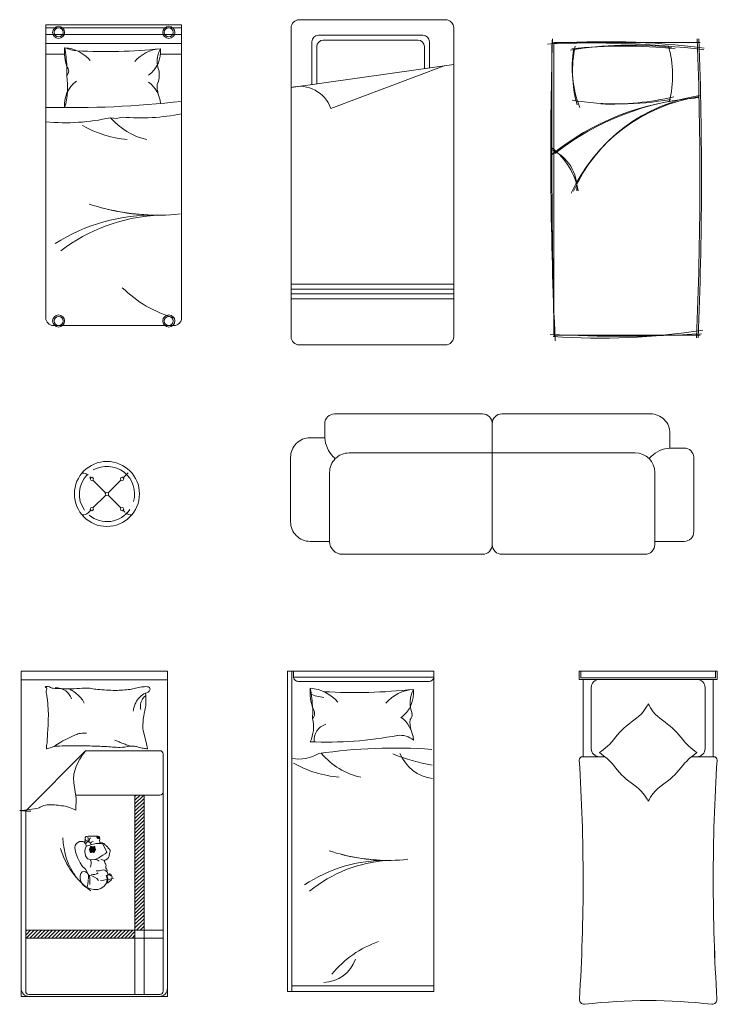
# Model space of a CAD drawing. Units: inches. Extents: x -17 to 1735, y -531 to 60.
# Tile 27 of 27: x 1734.8647 to 1735.0336, y -150.4015 to -150.163. Entities that reach past the tile are written whole.
import ezdxf

# ---------------------------------------------------------------- set-up
doc = ezdxf.new("R2010")
doc.units = ezdxf.units.IN
doc.header["$MEASUREMENT"] = 0
doc.layers.add('A-FURN', color=242, linetype='Continuous', lineweight=18, true_color=0xcd2027)
pattern_1 = [(315, (86.7872822, 39.0477945), (0.00194454365, 0.00194454365), [])]

# ---------------------------------------------------------------- blocks, each defined once
blk = doc.blocks.new('childrens_room_2')
h = blk.add_hatch()
h.set_pattern_fill('ANSI31', color=256, scale=0.005, angle=-90, style=0)
h.set_pattern_definition([(45, (74.756955, 52.19314), (-0.01122532, 0.01122532), [])])
h.paths.add_polyline_path([(75.7484, 49.9124), (75.6924, 49.9124), (75.6924, 50.7433), (75.7484, 50.7433)])
h.paths.add_polyline_path([(75.6924, 49.9124), (75.6924, 49.8634), (75.0203, 49.8634), (75.0203, 49.9124)])
h = blk.add_hatch()
h.set_pattern_fill('ANSI31', color=256, scale=0.022, angle=-90, style=0)
h.set_pattern_definition(pattern_1)
h.paths.add_polyline_path([(75.4756, 50.4754), (75.4753, 50.4804), (75.4736, 50.4848), (75.4694, 50.4881), (75.4661, 50.4896), (75.4574, 50.4905, 0.479357)])
h = blk.add_hatch()
h.set_pattern_fill('ANSI31', color=256, scale=0.022, angle=-90, style=0)
h.set_pattern_definition(pattern_1)
h.paths.add_polyline_path([(75.4157, 50.4038), (75.4153, 50.3984), (75.4172, 50.3931), (75.4208, 50.39), (75.425, 50.39), (75.431, 50.3928), (75.4354, 50.3938), (75.4375, 50.3921), (75.4403, 50.3907), (75.4436, 50.3921), (75.4442, 50.3948), (75.4443, 50.3978), (75.4455, 50.4018), (75.4489, 50.407), (75.4494, 50.4084), (75.446, 50.4144), (75.445, 50.417), (75.4457, 50.4212), (75.4461, 50.4241), (75.4435, 50.4269), (75.4407, 50.4259), (75.4383, 50.4231), (75.4332, 50.4237), (75.4242, 50.4273), (75.4199, 50.4264), (75.4193, 50.4235), (75.4187, 50.4213), (75.4164, 50.4195), (75.4165, 50.4173), (75.4153, 50.4135), (75.4128, 50.4109), (75.4115, 50.4095), (75.4136, 50.4078)])
for p, q in [((75.9793, 55.4814), (75.144, 55.4814)), ((75.144, 55.4814), (75.144, 53.6781)), ((75.9793, 55.4814), (75.9793, 53.6781)), ((76.7025, 55.5128), (77.6025, 55.5128)), ((75.9793, 55.4628), (75.144, 55.4628)), ((75.9793, 55.4225), (75.144, 55.4225)), ((76.6525, 53.5628), (76.6525, 55.4628)), ((77.6525, 53.5628), (77.6525, 55.4628)), ((75.9793, 55.3673), (75.144, 55.3673)), ((76.7804, 55.3772), (76.7804, 55.1146)), ((77.4628, 55.4172), (76.8204, 55.4172)), ((77.4328, 55.3872), (76.8504, 55.3872)), ((77.5028, 55.2164), (77.5028, 55.3772)), ((78.2687, 55.3728), (79.1687, 55.3728)), ((78.2687, 53.5728), (78.2687, 55.3728)), ((75.2595, 55.3013), (75.144, 55.3013)), ((75.9793, 55.3013), (75.8487, 55.3013)), ((76.8104, 55.3472), (76.8104, 55.1188)), ((77.4728, 55.2122), (77.4728, 55.3472)), ((77.6525, 55.2375), (76.6525, 55.0966)), ((76.8961, 54.9672), (77.5948, 55.2294)), ((76.6525, 53.8862), (77.6525, 53.8862)), ((76.6525, 53.8562), (77.6525, 53.8562)), ((76.6525, 53.8262), (77.6525, 53.8262)), ((76.6525, 53.7962), (77.6525, 53.7962)), ((75.1904, 53.6317), (75.9329, 53.6317)), ((79.1687, 53.5728), (78.2687, 53.5728)), ((77.6025, 53.5128), (76.7025, 53.5128)), ((76.8595, 53.0278), (76.8595, 52.941)), ((77.8894, 53.0282), (77.8894, 52.2842)), ((77.8894, 52.2842), (77.8894, 53.0282)), ((76.8599, 52.941), (76.7694, 52.941)), ((78.9826, 52.8777), (78.9826, 52.9682)), ((76.9245, 52.8126), (76.9123, 52.8249)), ((77.0094, 52.8478), (77.8894, 52.8482)), ((77.8894, 52.8482), (78.7694, 52.8482)), ((78.8542, 52.813), (78.8665, 52.8253)), ((75.4201, 52.6953), (75.4145, 52.7009)), ((75.6201, 52.6953), (75.6509, 52.7262)), ((76.8894, 52.3038), (76.8894, 52.7278)), ((78.8894, 52.7282), (78.8894, 52.3038)), ((75.51, 52.6054), (75.4343, 52.6812)), ((75.5272, 52.6024), (75.6059, 52.6812)), ((75.4343, 52.5095), (75.513, 52.5883)), ((75.6059, 52.5095), (75.5301, 52.5853)), ((75.4046, 52.4798), (75.4201, 52.4954)), ((75.631, 52.4844), (75.6201, 52.4954)), ((76.7694, 52.3038), (76.8894, 52.3038)), ((78.8894, 52.2842), (78.8894, 52.3038)), ((77.4337, 52.2242), (77.4534, 52.2242)), ((74.9919, 51.5044), (74.9919, 49.5044)), ((75.8919, 51.5044), (74.9919, 51.5044)), ((75.8919, 49.5044), (75.8919, 51.5044)), ((76.6309, 49.5344), (76.6309, 51.5044)), ((76.6309, 51.5044), (77.5309, 51.5044)), ((76.6579, 49.5344), (76.6579, 51.5044)), ((77.5309, 51.5044), (77.5309, 49.5344)), ((75.8919, 51.452), (74.9919, 51.452)), ((76.6669, 51.4694), (77.5309, 51.4694)), ((78.4985, 51.4044), (78.4985, 51.0294)), ((79.1985, 51.4044), (79.1985, 51.0294)), ((75.3892, 51.0159), (75.0203, 50.6461)), ((75.3892, 51.0159), (75.8461, 51.0159)), ((75.8661, 50.9959), (75.8661, 49.5366)), ((78.4449, 50.9794), (78.582, 50.9794)), ((79.1151, 50.9794), (79.2522, 50.9794)), ((75.8461, 50.7433), (75.3274, 50.7433)), ((75.0203, 49.5366), (75.0203, 50.6461)), ((75.8661, 49.9124), (75.0203, 49.9124)), ((75.8661, 49.8634), (75.0203, 49.8634)), ((77.5309, 49.5694), (76.6579, 49.5694)), ((74.9919, 49.5044), (75.8919, 49.5044)), ((75.8461, 49.5166), (75.0403, 49.5166)), ((77.5309, 49.5344), (76.6309, 49.5344))]:
    blk.add_line(p, q)
for points in [[(75.144, 54.8843, 0.078314), (75.5425, 54.9102, 0.174082), (75.6138, 54.9142, 0.074189), (75.9793, 54.9344)], [(78.8294, 52.2242), (77.9494, 52.2242, -0.414214), (77.8894, 52.2842, -0.414214), (77.8294, 52.2242), (77.4534, 52.2242), (77.4534, 52.2242, -0.414214), (77.4534, 52.2242), (76.9678, 52.2242, -0.404299), (76.8894, 52.3038), (76.7694, 52.3038, -0.414214), (76.6494, 52.4238), (76.6494, 52.821, -0.414214), (76.7694, 52.941), (76.8595, 52.941), (76.8595, 53.0278, -0.409533), (76.9195, 53.0882), (77.8294, 53.0882, -0.414482), (77.8894, 53.0282, -0.414214), (77.9494, 53.0882), (78.8626, 53.0882, -0.414214), (78.9826, 52.9682), (78.9826, 52.878), (79.0694, 52.878, -0.394315), (79.1292, 52.8221), (79.1294, 52.3638, -0.41421), (79.0694, 52.3038), (78.8894, 52.3038), (78.8894, 52.2842, -0.414214), (78.8294, 52.2242, -2.414214)], [(76.6669, 51.5044), (76.6669, 51.4726, 0.414214), (76.6969, 51.4426), (77.5009, 51.4426, 0.414214), (77.5309, 51.4726)], [(79.2522, 50.9794), (79.2485, 50.9794), (79.2485, 51.4544), (79.2735, 51.4544), (79.2735, 51.5044), (78.4235, 51.5044), (78.4235, 51.4544), (78.4485, 51.4544), (78.4485, 50.9794), (78.4449, 50.9794, 0.433007), (78.4249, 50.9581, -0.031616), (78.4257, 49.4879, 0.44677), (78.457, 49.456, -0.059749), (79.24, 49.456, 0.44677), (79.2714, 49.4879, -0.031616), (79.2722, 50.9581, 0.433007), (79.2522, 50.9794), (79.2485, 50.9794)], [(75.7568, 51.3708, 0.263368), (75.7848, 51.3896, 0.494818), (75.7756, 51.4083, 0.049225), (75.7579, 51.4101, 0.036831), (75.7343, 51.4083, 0.031893), (75.6963, 51.4002, -0.035782), (75.6624, 51.3932, -0.032941), (75.5727, 51.3873, -0.026564), (75.4615, 51.3932, -0.017905), (75.424, 51.3986, 0.033397), (75.4038, 51.4008, 0.03204), (75.3667, 51.4001, -0.018442), (75.3024, 51.3971, -0.010837), (75.2376, 51.3978, -0.014624), (75.1897, 51.4008, -0.111249), (75.1671, 51.4081, 0.153708), (75.1503, 51.4121, 0.076444), (75.1428, 51.4104, 0.215512), (75.1409, 51.4083, 0.585858), (75.1435, 51.4053, -0.363489), (75.1484, 51.4027, -0.191716), (75.1484, 51.3912, 0.129675), (75.1465, 51.3746, 0.01735), (75.1495, 51.3577, -0.019326), (75.1521, 51.3427, -0.018818), (75.1587, 51.2743, -0.021828), (75.1596, 51.215, -0.006204), (75.1583, 51.1812, -0.001963), (75.1521, 51.0743, -0.028341), (75.1479, 51.0382, 0.117014), (75.1484, 51.0293, 0.36606), (75.1498, 51.0283, 0.03973), (75.1634, 51.0311, 0.048309), (75.1771, 51.0366, -0.062981), (75.1878, 51.0405, -0.04058), (75.2112, 51.0439, -0.014345), (75.2779, 51.0461, -0.005484), (75.4034, 51.0454, -0.007153), (75.4995, 51.0424, -0.008762), (75.5421, 51.0397, 0.008153), (75.5878, 51.0368, 0.06251), (75.6449, 51.0412, -0.078669), (75.6905, 51.0432, -0.047825), (75.7129, 51.0385, 0.034494), (75.7437, 51.0311, 0.023571), (75.769, 51.0281, 0.510228), (75.7699, 51.0293), (75.7624, 51.0593), (75.7418, 51.1419, -0.073041), (75.7398, 51.1614, -0.023305), (75.7455, 51.2225, -0.018299), (75.7496, 51.2454, 0.01097), (75.7569, 51.2834, 0.042281), (75.7599, 51.3177, 0.027201), (75.7569, 51.3711)], [(75.201, 51.4027, -0.088153), (75.2355, 51.3992, -0.088153), (75.2667, 51.3839, -0.077547), (75.2883, 51.3623, -0.077547), (75.3024, 51.3351)], [(75.2829, 51.397, -0.027842), (75.3067, 51.3864, -0.048685), (75.3193, 51.3783, -0.023666), (75.3472, 51.3539, -0.031223), (75.3662, 51.3333, -0.046801), (75.3713, 51.3256, -0.023191), (75.3794, 51.3089)], [(75.757, 51.3708, 0.077379), (75.7222, 51.3455, 0.077379), (75.6967, 51.3107, 0.047525), (75.6868, 51.2861, 0.047525), (75.6817, 51.2601)], [(75.7585, 51.3548, 0.05369), (75.7442, 51.3418, 0.070312), (75.7361, 51.3295, 0.015448), (75.7324, 51.321, 0.013244), (75.7286, 51.3107, 0.082127), (75.7256, 51.2927, 0.064164), (75.7286, 51.2695)], [(75.1972, 51.0424, -0.016108), (75.2361, 51.0686, -0.024599), (75.2629, 51.0837, -0.009477), (75.312, 51.107, -0.015937), (75.3418, 51.1193, -0.072521), (75.3581, 51.1229, -0.033339), (75.3944, 51.1231)], [(75.6664, 51.0439, -0.009729), (75.6391, 51.053, -0.009729), (75.6122, 51.063, -0.007971), (75.5905, 51.0721, -0.007971), (75.569, 51.0818)], [(75.3892, 51.0159, 0.085272), (75.3259, 50.9058, 0.124044), (75.3167, 50.8182), (75.3304, 50.7228), (75.3286, 50.6503)], [(76.6579, 50.9684, 0.174518), (76.8222, 50.998, -0.055694), (77.517, 51.0241)], [(75.3286, 50.6503, 0.027362), (75.2901, 50.6667, 0.040834), (75.2629, 50.6741, 0.038441), (75.1753, 50.6837, 0.076528), (75.1312, 50.6783, 0.103649), (75.1036, 50.6639, -0.026469), (74.9835, 50.6474, -0.024037), (75.0514, 50.6436, -0.052315), (75.0203, 50.6461)]]:
    blk.add_lwpolyline(points, format="xyb")
for points in [[(78.4235, 51.4544), (79.2735, 51.4544), (79.2735, 51.5044), (78.4235, 51.5044)], [(78.4335, 51.4644), (79.2635, 51.4644), (79.2635, 51.5044), (78.4335, 51.5044)]]:
    blk.add_lwpolyline(points, close=True)
for points in [[(79.2485, 50.9794), (79.2485, 51.4544), (78.4485, 51.4544), (78.4485, 50.9794)], [(75.6924, 49.5166), (75.6924, 50.7433)], [(75.7484, 49.5166), (75.7484, 50.7433)], [(75.4495, 50.4907), (75.436, 50.4914), (75.4203, 50.4904), (75.4036, 50.4898), (75.3986, 50.4892), (75.3926, 50.4889), (75.3864, 50.4823), (75.386, 50.476), (75.3873, 50.4713), (75.3842, 50.4665), (75.3854, 50.4621), (75.382, 50.454), (75.3779, 50.4546), (75.3722, 50.4577), (75.3521, 50.4571), (75.3405, 50.4511), (75.3333, 50.4449), (75.3254, 50.4326), (75.3235, 50.4197), (75.3264, 50.3946), (75.338, 50.359), (75.3556, 50.3273), (75.3703, 50.3034), (75.3857, 50.2905), (75.3892, 50.288), (75.3989, 50.2691), (75.3992, 50.2672), (75.3974, 50.2654), (75.3879, 50.2716), (75.381, 50.2735), (75.3675, 50.272), (75.3603, 50.2613), (75.3555, 50.2467), (75.3548, 50.229), (75.3596, 50.2113), (75.3725, 50.1916), (75.3908, 50.176), (75.4017, 50.1719), (75.4078, 50.1712), (75.4214, 50.1658), (75.4397, 50.1631), (75.4642, 50.1631), (75.4832, 50.1685), (75.5022, 50.1835), (75.5165, 50.2018), (75.526, 50.2039), (75.547, 50.2188), (75.5518, 50.2372), (75.5443, 50.2569), (75.5375, 50.2582), (75.5308, 50.2525), (75.5289, 50.252), (75.5261, 50.2586), (75.5239, 50.263), (75.5228, 50.2642), (75.5217, 50.27), (75.5203, 50.2719), (75.5214, 50.2813), (75.5169, 50.2902), (75.5139, 50.293), (75.5136, 50.3049), (75.515, 50.3102), (75.5106, 50.3204), (75.5086, 50.3215), (75.5078, 50.3309), (75.5039, 50.3376), (75.5061, 50.342), (75.5128, 50.3453), (75.5233, 50.3506), (75.5305, 50.3589), (75.5327, 50.3678), (75.5344, 50.3728), (75.5349, 50.3805), (75.5361, 50.3864), (75.5394, 50.3933), (75.5408, 50.3972), (75.5405, 50.4041), (75.5336, 50.4127), (75.5297, 50.4138), (75.5264, 50.4215), (75.5233, 50.426), (75.5194, 50.4274), (75.5175, 50.4296), (75.5158, 50.4321), (75.51, 50.4348), (75.5086, 50.436), (75.5086, 50.4379), (75.5031, 50.4432), (75.5006, 50.4457), (75.4962, 50.4454), (75.4917, 50.449), (75.4879, 50.4487), (75.4807, 50.4493), (75.4773, 50.4501), (75.476, 50.4509), (75.4766, 50.4526), (75.4769, 50.4574), (75.4751, 50.461), (75.4749, 50.4631), (75.4758, 50.4719), (75.4753, 50.4804), (75.4736, 50.4848), (75.4694, 50.4881), (75.4661, 50.4896), (75.4532, 50.4909), (75.4495, 50.4907)], [(75.4954, 50.4409), (75.5077, 50.4188), (75.5192, 50.3914), (75.5099, 50.3825), (75.494, 50.3728), (75.4662, 50.3551), (75.4463, 50.3472), (75.4251, 50.345), (75.4004, 50.3512), (75.3889, 50.3693), (75.384, 50.3954), (75.3863, 50.4148), (75.3942, 50.4289), (75.4269, 50.4387), (75.453, 50.4444), (75.4803, 50.4453), (75.4954, 50.4409)], [(75.4494, 50.4084), (75.446, 50.4144), (75.445, 50.417), (75.4457, 50.4212), (75.4461, 50.4241), (75.4435, 50.4269), (75.4407, 50.4259), (75.4383, 50.4231), (75.4332, 50.4237), (75.4242, 50.4273), (75.4199, 50.4264), (75.4193, 50.4235), (75.4187, 50.4213), (75.4164, 50.4195), (75.4165, 50.4173), (75.4153, 50.4135), (75.4128, 50.4109), (75.4115, 50.4095), (75.4136, 50.4078), (75.4157, 50.4038), (75.4153, 50.3984), (75.4172, 50.3931), (75.4208, 50.39), (75.425, 50.39), (75.431, 50.3928), (75.4354, 50.3938), (75.4375, 50.3921), (75.4403, 50.3907), (75.4436, 50.3921), (75.4442, 50.3948), (75.4443, 50.3978), (75.4455, 50.4018), (75.4489, 50.407), (75.4494, 50.4084)]]:
    blk.add_lwpolyline(points)
for centre, radius in [((75.2229, 55.435), 0.0371), ((75.2229, 55.435), 0.0278), ((75.9004, 55.435), 0.0371), ((75.9004, 55.435), 0.0278), ((75.2229, 53.6596), 0.0371), ((75.2229, 53.6596), 0.0278), ((75.9004, 53.6596), 0.0371), ((75.9004, 53.6596), 0.0278), ((75.5201, 52.5954), 0.2), ((75.4272, 52.6883), 0.01), ((75.613, 52.6883), 0.01), ((75.5201, 52.5954), 0.01), ((75.4272, 52.5025), 0.01), ((75.613, 52.5025), 0.01)]:
    blk.add_circle(centre, radius)
for centre, radius, start, end in [((76.7025, 55.4628), 0.05, 90, 180), ((77.6025, 55.4628), 0.05, 0, 90), ((76.8204, 55.3772), 0.04, 90, 180), ((76.8504, 55.3472), 0.04, 90, 180), ((77.4328, 55.3472), 0.04, 0, 90), ((77.4628, 55.3772), 0.04, 0, 90), ((78.5913, 50.8189), 4.5588, 82.42637, 94.55161), ((78.5011, 49.6503), 5.7195, 83.0717, 92.72063), ((102.953, 54.6963), 24.7034, 178.37753, 182.68762), ((142.1352, 54.9109), 63.8797, 179.573644, 181.208723), ((56.1732, 54.5417), 22.9932, 357.54182, 2.12882), ((56.1732, 54.5417), 23.0032, 357.54182, 2.12882), ((75.5453, 55.3172), 0.2863, 175.30484, 198.69419), ((75.3647, 55.5935), 0.2736, 247.51785, 264.26696), ((75.2441, 55.1139), 0.2274, 40.4189, 85.9871), ((73.7608, 55.0981), 1.5188, 4.80985, 9.18918), ((75.5117, 58.4538), 3.1374, 266.81337, 276.16021), ((75.8643, 55.1077), 0.2274, 94.0129, 139.5811), ((75.669, 55.316), 0.1804, 306.5711, 5.88998), ((75.9929, 55.2569), 0.164, 151.77364, 201.69827), ((78.7416, 53.0702), 2.286, 83.69688, 99.35881), ((78.6932, 52.3041), 3.0464, 83.94088, 95.93515), ((79.0436, 55.2168), 0.6622, 169.79049, 201.55888), ((79.1653, 55.1958), 0.7819, 168.56961, 195.27012), ((78.3558, 55.1693), 0.6428, 345.48198, 16.58826), ((75.2435, 55.1977), 0.0414, 314.4736, 42.17134), ((73.0827, 55.2679), 2.1921, 357.39054, 358.88764), ((75.6858, 55.1758), 0.156, 337.01696, 7.53676), ((75.4394, 54.9904), 0.1804, 126.5711, 185.88998), ((74.8178, 55.0985), 0.46, 344.0243, 8.70709), ((75.669, 54.9843), 0.1804, 4.31813, 53.4289), ((75.9991, 55.1007), 0.1702, 175.22328, 196.23004), ((76.7043, 54.9001), 0.2032, 19.27951, 104.76299), ((75.2957, 61.0539), 6.082, 268.57082, 276.45367), ((79.2465, 53.4559), 1.5775, 94.14563, 129.02089), ((79.2814, 53.412), 1.6265, 94.18593, 128.21496), ((79.3165, 54.015), 1.0355, 98.91724, 155.46246), ((78.6697, 56.7642), 1.7696, 260.58531, 280.2821), ((79.3129, 54.0449), 1.0119, 98.39844, 155.88807), ((78.6184, 56.6764), 1.6826, 267.95445, 283.33938), ((75.5045, 53.3317), 1.6584, 97.85852, 98.47626), ((75.2441, 55.1987), 0.2274, 274.0129, 278.34166), ((75.8605, 55.1841), 0.4198, 220.73328, 256.96719), ((75.7087, 55.4543), 0.6823, 240.14078, 264.51099), ((78.1507, 54.4748), 0.2599, 356.64662, 66.65295), ((77.9988, 54.3854), 0.4254, 10.16482, 52.268), ((75.8487, 55.7499), 1.4398, 252.27047, 269.13024), ((75.8269, 55.5836), 1.2733, 255.03258, 276.43831), ((75.8025, 53.1895), 1.1211, 88.75448, 122.44857), ((75.8891, 53.2381), 1.074, 93.31876, 127.41471), ((76.1443, 54.4045), 0.7565, 225.55548, 253.7707), ((75.1904, 53.6781), 0.0464, 180, 270), ((75.9329, 53.6781), 0.0464, 270, 0), ((78.5471, 57.6422), 4.0883, 266.02934, 278.96409), ((76.7025, 53.5628), 0.05, 180, 270), ((77.6025, 53.5628), 0.05, 270, 0), ((78.6779, 61.5696), 8.0041, 266.89864, 273.56403), ((75.5201, 52.5954), 0.17, 344.03296, 119.71985), ((75.5201, 52.5954), 0.17, 135.42029, 215.97163), ((75.3738, 52.6824), 0.0419, 42.82742, 99.74562), ((75.503, 52.6011), 0.0083, 347.80192, 31.53697), ((75.5396, 52.5905), 0.0108, 179.91033, 208.61328), ((75.3738, 52.5083), 0.0419, 260.25438, 317.17258), ((75.5201, 52.5954), 0.17, 229.841, 326.08002), ((75.6664, 52.5083), 0.0419, 222.82742, 279.74562), ((78.5485, 51.4044), 0.05, 90, 180), ((79.1485, 51.4044), 0.05, 0, 90), ((77.0781, 51.3748), 0.3085, 175.30484, 198.69419), ((75.1553, 51.1387), 1.6364, 4.80985, 9.18918), ((76.7535, 51.1557), 0.245, 40.4189, 85.9871), ((76.8834, 51.6374), 0.2948, 247.51785, 264.26696), ((77.0419, 54.7542), 3.3803, 266.81337, 276.16021), ((77.4217, 51.149), 0.245, 94.0129, 139.5811), ((77.2113, 51.3735), 0.1943, 306.5711, 5.88998), ((77.5603, 51.3098), 0.1767, 151.77364, 201.69827), ((76.7528, 51.246), 0.0446, 314.4736, 42.17134), ((74.4247, 51.3217), 2.3618, 357.39054, 358.88764), ((77.3634, 51.2349), 0.034, 307.61433, 16.28017), ((76.5848, 51.1619), 0.206, 333.80176, 14.68402), ((77.2113, 51.0672), 0.1943, 4.31813, 53.4289), ((77.5669, 51.1927), 0.1834, 175.22328, 196.23004), ((76.8943, 51.0822), 0.1005, 106.29058, 186.59246), ((76.8707, 53.382), 2.3132, 267.49728, 280.89487), ((77.3213, 50.9766), 0.1345, 51.46896, 95.71894), ((75.8461, 50.9959), 0.02, 0, 90), ((78.5485, 51.0294), 0.05, 180, 270), ((79.1485, 51.0294), 0.05, 270, 0), ((77.0193, 51.5842), 0.7351, 241.35539, 264.51099), ((77.1829, 51.2931), 0.4523, 220.73328, 256.96719), ((77.7873, 52.3166), 1.4152, 248.91606, 259.13002), ((77.5533, 51.0927), 0.2498, 202.22848, 262.85937), ((78.4449, 50.9594), 0.02, 90, 183.6518), ((66.811, 50.2169), 11.6375, 356.40829, 3.6518), ((90.886, 50.2169), 11.6375, 176.3482, 183.59171), ((79.2522, 50.9594), 0.02, 356.3482, 90), ((75.8461, 50.7633), 0.02, 270, 0), ((75.6808, 50.4898), 0.4315, 181.3671, 216.20735), ((75.3593, 50.4268), 0.0334, 2.14976, 56.17832), ((75.3953, 50.449), 0.0128, 86.19942, 139.06656), ((75.4077, 50.4378), 0.0188, 115.21484, 159.80112), ((75.3835, 50.4189), 0.0447, 30.58858, 73.49123), ((75.3615, 50.4709), 0.0431, 344.84219, 17.23973), ((75.4376, 50.4582), 0.0279, 129.74508, 181.73372), ((75.4384, 50.4355), 0.0218, 99.96051, 151.84303), ((75.4726, 50.4902), 0.0152, 179.09874, 281.54292), ((75.7102, 50.5592), 0.4972, 196.86297, 234.46246), ((77.2654, 51.5819), 1.241, 252.27047, 269.13024), ((75.3803, 50.3234), 0.043, 327.51496, 27.23561), ((75.444, 50.306), 0.0412, 46.79486, 86.71559), ((75.4409, 50.2001), 0.1537, 65.34145, 74.49126), ((77.2271, 49.466), 0.8752, 88.72565, 124.14447), ((77.2985, 49.5044), 0.8382, 93.5571, 129.40281), ((77.2465, 51.4385), 1.0975, 255.03258, 276.43831), ((75.4555, 50.4129), 0.1357, 269.28478, 284.50888), ((75.4981, 50.2552), 0.0277, 37.10802, 108.24352), ((75.2967, 50.2148), 0.1077, 337.68374, 4.59021), ((75.4403, 50.2845), 0.0458, 203.4063, 230.89091), ((75.3353, 50.2361), 0.0716, 352.96919, 16.79875), ((75.2773, 50.2141), 0.1386, 351.00842, 14.55404), ((75.4051, 50.1708), 0.0784, 35.92195, 85.40551), ((75.4384, 50.2916), 0.0377, 247.42864, 316.0363), ((75.3609, 51.3141), 1.1027, 276.25277, 280.37834), ((75.5175, 50.2626), 0.0134, 263.95418, 321.01796), ((75.4856, 50.2225), 0.0407, 331.14901, 41.38363), ((75.4513, 50.2251), 0.0692, 340.33191, 20.51812), ((75.5304, 50.2371), 0.0162, 38.30312, 78.93742), ((77.397, 49.2401), 0.6361, 108.97703, 140.93858), ((76.8471, 49.8039), 0.2131, 271.60281, 340.57338), ((75.0418, 49.5544), 0.05, 180, 270), ((75.8419, 49.5544), 0.05, 270, 0), ((75.0403, 49.5366), 0.02, 180, 270), ((75.8461, 49.5366), 0.02, 270, 0), ((78.4556, 49.486), 0.03, 176.40829, 272.70295), ((79.2415, 49.486), 0.03, 267.29705, 3.59171), ((78.8485, 46.1915), 3.2879, 83.1614, 96.8386)]:
    blk.add_arc(centre, radius, start, end)
at = {"extrusion": (0, 0, -1)}
for centre, major_axis, start_param, end_param in [((77.0395, 52.9522), (-0.1273, -0.1273), 0, 0.723307), ((77.0094, 52.7278), (0.0849, -0.0849), 2.356194, 3.926991)]:
    blk.add_ellipse(centre, major_axis=major_axis, ratio=1, start_param=start_param, end_param=end_param, dxfattribs=at)
for centre, major_axis, start_param, end_param in [((78.9938, 52.698), (-0.1273, -0.1273), 3.989082, 4.712389), ((78.7694, 52.7282), (0.0849, -0.0849), 0.785398, 2.356194)]:
    blk.add_ellipse(centre, major_axis=major_axis, ratio=1, start_param=start_param, end_param=end_param)
for points in [[(78.5488, 51.0047), (78.5659, 51.0173), (78.6232, 51.0595), (78.6908, 51.1657), (78.8035, 51.2251), (78.839, 51.2877), (78.8485, 51.3044)], [(79.1483, 51.0047), (79.1312, 51.0173), (79.0739, 51.0595), (79.0063, 51.1657), (78.8936, 51.2251), (78.8581, 51.2877), (78.8485, 51.3044)], [(78.5488, 51.0047), (78.5659, 50.9921), (78.6232, 50.9499), (78.6908, 50.8437), (78.8035, 50.7843), (78.839, 50.7217), (78.8485, 50.705)], [(79.1483, 51.0047), (79.1312, 50.9921), (79.0739, 50.9499), (79.0063, 50.8437), (78.8936, 50.7843), (78.8581, 50.7217), (78.8485, 50.705)]]:
    blk.add_open_spline(points, degree=3, knots=[0, 0, 0, 0, 0.0634005, 0.2125031, 0.3690804, 0.426269, 0.426269, 0.426269, 0.426269])

msp = doc.modelspace()

# ---------------------------------------------------------------- block references
at = {"layer": 'A-FURN', "xscale": 0.0393700787401575, "yscale": 0.0393700787401575, "zscale": 0.0393700787401575}
msp.add_blockref('childrens_room_2', (1731.9126, -152.34857), dxfattribs=at)

doc.saveas('drawing.dxf')
